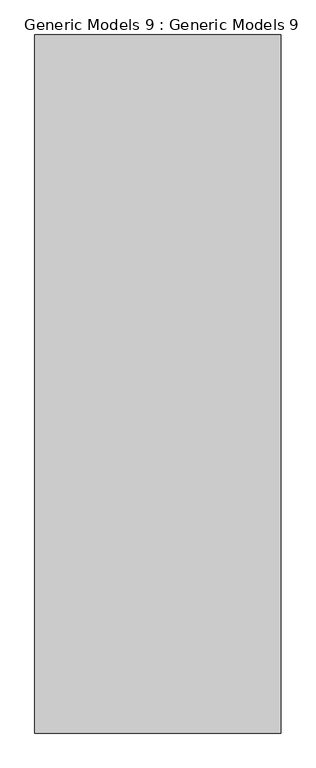
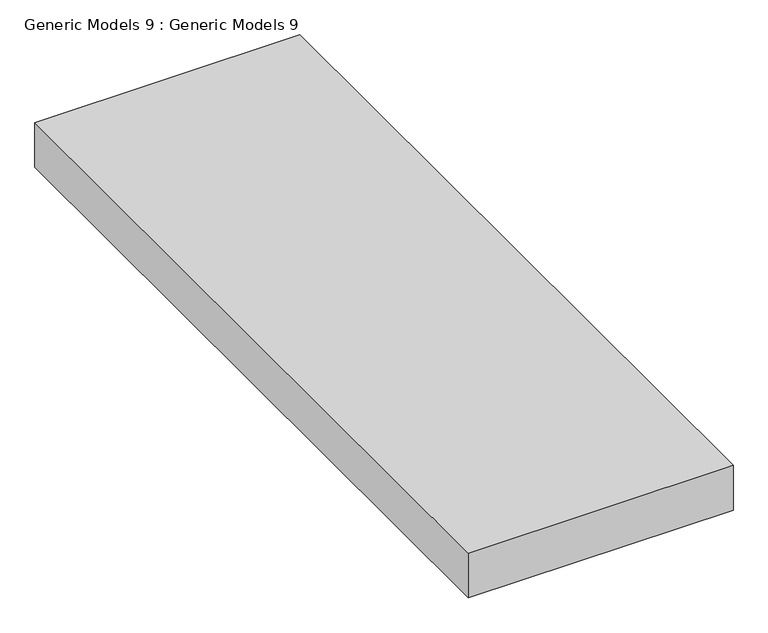
"""IFC4 building model written with IfcOpenShell, lengths in millimetres: proxy geometry, Generic Models 9 : Generic Models 9."""

from ifc_helpers import new_model, si_unit, frame, origin, place, context, project, spatial, polyline, outline, extrude, source, transform, mapped, element, save


def generic_models_9_generic_models_9_e403c41d(model_context):
    return source(origin(), model_context, "Body", "SweptSolid", [
        extrude(outline(polyline([(-22696.5161422, -470.8893556), (-21845.6161422, -470.8893556), (-21845.6161422, -2882.023242), (-22696.5161422, -2882.023242), (-22696.5161422, -470.8893556)])), frame((0.0, 0.0, 2524.5687713), z_axis=(0.0, 0.0, 1.0), x_axis=(1.0, 0.0, 0.0)), (0.0, 0.0, 1.0), 152.4),
    ])


if __name__ == "__main__":
    model = new_model("IFC4")
    model_context = context("Model", 3, world=origin())
    ifc_project = project(units=[si_unit("LENGTHUNIT", "METRE", prefix="MILLI")], contexts=[model_context])
    site = spatial("IfcSite", under=ifc_project)
    building = spatial("IfcBuilding", under=site)
    placement = place(None, origin())
    generic_models_9_generic_models_9_shape = generic_models_9_generic_models_9_e403c41d(model_context)
    element("IfcBuildingElementProxy", 1, Name="Generic Models 9 : Generic Models 9", ObjectType="Generic Models 9 : Generic Models 9", at=placement, inside=building, context=model_context, shape_type="MappedRepresentation", body=[
        mapped(generic_models_9_generic_models_9_shape, transform((0.0, 0.0, 0.0), x_axis=(1.0, 0.0, 0.0), y_axis=(0.0, 1.0, 0.0), z_axis=(0.0, 0.0, 1.0))),
    ])
    save(model, "model.ifc")
